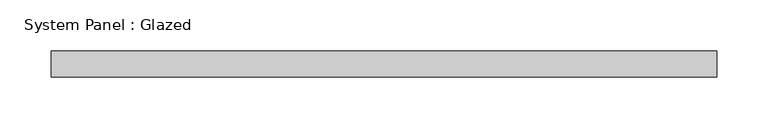
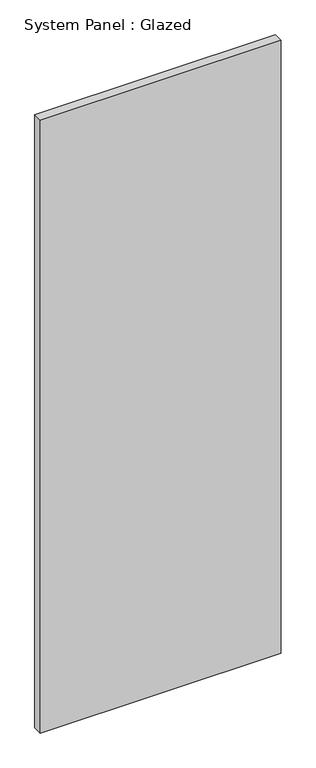
"""IFC4 building model written with IfcOpenShell, lengths in millimetres: plate geometry, System Panel : Glazed."""

from ifc_helpers import new_model, si_unit, origin, origin_with_axes, place, context, project, spatial, polyline, outline, extrude, source, transform, mapped, element, save


def system_panel_glazed_64df1ed2(model_context):
    return source(origin(), model_context, "Body", "SweptSolid", [
        extrude(outline(polyline([(323.85, 19.05), (-323.85, 19.05), (-323.85, 44.45), (323.85, 44.45), (323.85, 19.05)])), origin_with_axes(), (0.0, 0.0, 1.0), 1741.0529055),
    ])


if __name__ == "__main__":
    model = new_model("IFC4")
    model_context = context("Model", 3, world=origin())
    ifc_project = project(units=[si_unit("LENGTHUNIT", "METRE", prefix="MILLI")], contexts=[model_context])
    site = spatial("IfcSite", under=ifc_project)
    building = spatial("IfcBuilding", under=site)
    placement = place(None, origin())
    system_panel_glazed_shape = system_panel_glazed_64df1ed2(model_context)
    element("IfcPlate", 1, ObjectType="System Panel : Glazed", at=placement, inside=building, context=model_context, shape_type="MappedRepresentation", body=[
        mapped(system_panel_glazed_shape, transform((0.0, 0.0, 0.0), x_axis=(1.0, 0.0, 0.0), y_axis=(0.0, 1.0, 0.0), z_axis=(0.0, 0.0, 1.0))),
    ])
    save(model, "model.ifc")

# Revit data of these elements
# Type "System Panel : Glazed"
#   Construction Type Id = "GSP4R"
#   Analytic Construction = "1/8 in Pilkington single glazing"
#   Visual Light Transmittance = 0.9
#   Solar Heat Gain Coefficient = 0.86
#   Heat Transfer Coefficient (U) = 1.18115 BTU/(h·ft²·°F)
#   Define Thermal Properties by = 1
# Element 1 (IfcPlate, "System Panel : Glazed")
#   Materials on its faces: "Glass"
# Materials
#   "Glass": class "Glass", colour RGB 0 128 192, transparency 0.75, Description = "Soda Lime Glass", Cost = 0
